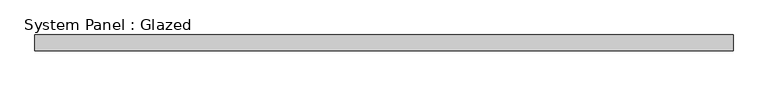
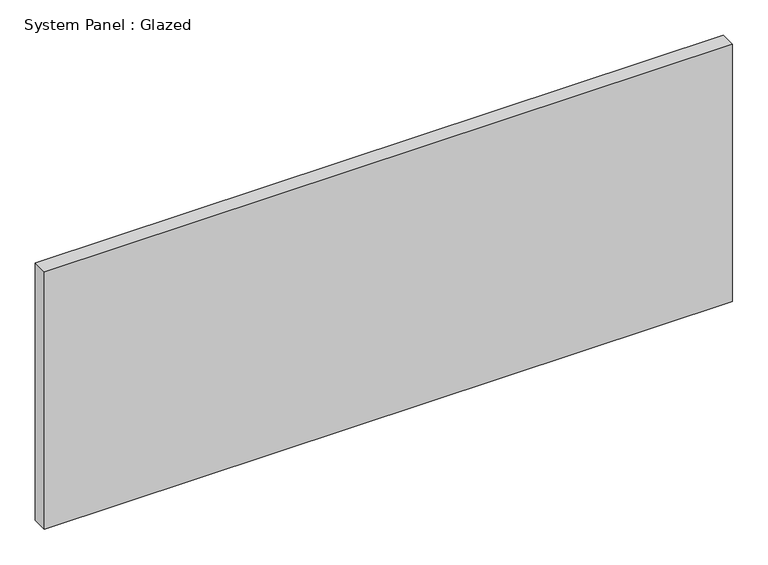
"""IFC4 building model written with IfcOpenShell, lengths in millimetres: plate geometry, System Panel : Glazed."""

from ifc_helpers import new_model, si_unit, origin, origin_with_axes, place, context, project, spatial, polyline, outline, extrude, source, transform, mapped, element, save


def system_panel_glazed_28d744da(model_context):
    return source(origin(), model_context, "Body", "SweptSolid", [
        extrude(outline(polyline([(561.975, -44.45), (-561.975, -44.45), (-561.975, -19.05), (561.975, -19.05), (561.975, -44.45)])), origin_with_axes(), (0.0, 0.0, 1.0), 444.5),
    ])


if __name__ == "__main__":
    model = new_model("IFC4")
    model_context = context("Model", 3, world=origin())
    ifc_project = project(units=[si_unit("LENGTHUNIT", "METRE", prefix="MILLI")], contexts=[model_context])
    site = spatial("IfcSite", under=ifc_project)
    building = spatial("IfcBuilding", under=site)
    placement = place(None, origin())
    system_panel_glazed_shape = system_panel_glazed_28d744da(model_context)
    element("IfcPlate", 1, ObjectType="System Panel : Glazed", at=placement, inside=building, context=model_context, shape_type="MappedRepresentation", body=[
        mapped(system_panel_glazed_shape, transform((0.0, 0.0, 0.0), x_axis=(1.0, 0.0, 0.0), y_axis=(0.0, 1.0, 0.0), z_axis=(0.0, 0.0, 1.0))),
    ])
    save(model, "model.ifc")

# Revit data of these elements
# Type "System Panel : Glazed"
#   Construction Type Id = "GSP4R"
#   Analytic Construction = "1/8 in Pilkington single glazing"
#   Visual Light Transmittance = 0.9
#   Solar Heat Gain Coefficient = 0.86
#   Heat Transfer Coefficient (U) = 1.18115 BTU/(h·ft²·°F)
#   Define Thermal Properties by = 1
# Element 1 (IfcPlate, "System Panel : Glazed")
#   Materials on its faces: "GARAGE PANEL"
# Materials
#   "GARAGE PANEL": class "Generic", colour RGB 120 120 120, transparency 0, Cost = 0
